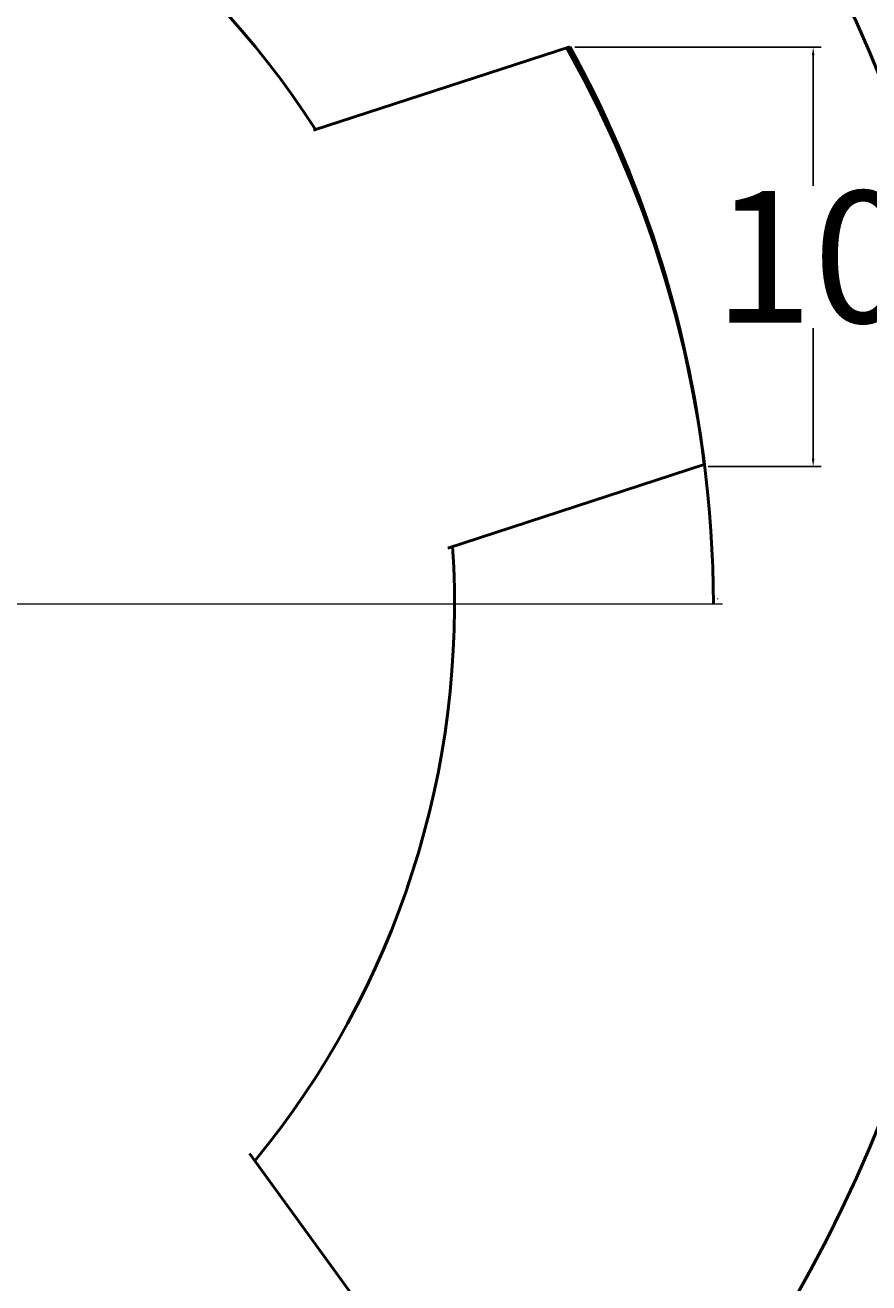
# Model space of a CAD drawing. Units: millimetres. Extents: x -50 to 109, y -46 to 152.
# Tile 6 of 18: x 9 to 29, y -22 to 6. Entities that reach past the tile are written whole.
import ezdxf

# ---------------------------------------------------------------- set-up
doc = ezdxf.new("R2010")
doc.units = ezdxf.units.MM
doc.header["$MEASUREMENT"] = 0
doc.linetypes.add('CENTER', pattern=[50.8, 31.75, -6.35, 6.35, -6.35])
for name, color, linetype, lineweight in [('M-CNTR', 1, 'CENTER', 18), ('M-DIMS', 2, 'Continuous', 25), ('M-OUTL', 7, 'Continuous', 50)]:
    doc.layers.add(name, color=color, linetype=linetype, lineweight=lineweight)
doc.styles.get("Standard").update_dxf_attribs({"font": 'arial.ttf'})
doc.dimstyles.get("Standard").update_dxf_attribs({"dimtxt": 0.18, "dimasz": 0.18, "dimexe": 0.18, "dimexo": 0.0625, "dimgap": 0.09, "dimtad": 0, "dimtih": 1, "dimtoh": 1, "dimdec": 4, "dimzin": 0, "dimdsep": 46, "dimtxsty": 'Standard', "dimcen": 0.09, "dimadec": 0, "dimazin": 0, "dimtfac": 1, "dimtdec": 4, "dimtofl": 0, "dimtmove": 0, "dimatfit": 3, "dimfxl": 1, "dimtolj": 1, "dimtzin": 0, "dimarcsym": 0})

# ---------------------------------------------------------------- blocks, each defined once
blk = doc.blocks.new('*U1')
for p, q in [((-5, 2.851), (-5, -3.294)), ((5, 2.824), (5, -3.323))]:
    blk.add_line(p, q)
blk.add_arc((-0.069, -22.677), 26, 78.7582, 100.9333)
blk = doc.blocks.new('*U2')
at = {"layer": 'M-OUTL', "color": 0, "linetype": 'ByBlock', "lineweight": -2, "transparency": 16777216}
for p, rotation in [((20.551, 0.185), 288), ((12.307, -25), 216)]:
    blk.add_blockref('*U1', p, dxfattribs=dict(at, rotation=rotation))
blk = doc.blocks.new('*U6')
at = {"layer": 'M-CNTR', "color": 0, "transparency": 16777216}
blk.add_line((5.2, 0), (26.12, 0), dxfattribs=at)
blk = doc.blocks.new('*D20')
at = {"layer": 'Defpoints', "color": 0, "transparency": 16777216}
for p in [(21.766, 5.813), (24.805, -3.739), (27.264, -3.739)]:
    blk.add_point(p, dxfattribs=at)
at = {"layer": 'M-DIMS', "color": 0, "lineweight": -2, "transparency": 16777216}
for p, q in [((21.828, 5.813), (27.444, 5.813)), ((27.264, 5.633), (27.264, 2.659)), ((27.264, -3.559), (27.264, -0.585)), ((24.868, -3.739), (27.444, -3.739))]:
    blk.add_line(p, q, dxfattribs=at)
at = {"layer": 'M-DIMS', "color": 0, "transparency": 16777216}
for points in [[(27.234, 5.633), (27.294, 5.633), (27.264, 5.813)], [(27.234, -3.559), (27.294, -3.559), (27.264, -3.739)]]:
    blk.add_solid(points, dxfattribs=at)
at = {"layer": 'M-DIMS', "color": 0, "transparency": 16777216, "insert": (27.264, 1.037), "char_height": 0.18, "attachment_point": 5}
blk.add_mtext('\\A1;{\\H16.66667x;10}', dxfattribs=at)
blk = doc.blocks.new('*D23')
at = {"layer": 'Defpoints', "color": 0, "transparency": 16777216}
for p in [(24.75, 12.317), (-26.598, -25.885)]:
    blk.add_point(p, dxfattribs=at)
at = {"layer": 'M-DIMS', "color": 0, "lineweight": -2, "transparency": 16777216}
for p, q in [((-1.014, -6.784), (-0.834, -6.784)), ((-0.924, -6.874), (-0.924, -6.694)), ((-30.604, -28.865), (-26.742, -25.992)), ((-30.784, -28.865), (-30.604, -28.865))]:
    blk.add_line(p, q, dxfattribs=at)
at = {"layer": 'M-DIMS', "color": 0, "transparency": 16777216}
blk.add_solid([(-26.76, -25.968), (-26.724, -26.016), (-26.598, -25.885)], dxfattribs=at)
at = {"layer": 'M-DIMS', "color": 0, "transparency": 16777216, "insert": (-34.648, -28.865), "char_height": 0.18, "attachment_point": 5}
blk.add_mtext('\\A1;{\\H16.66667x;%%C64}', dxfattribs=at)
blk = doc.blocks.new('*D29')
at = {"layer": 'Defpoints', "color": 0, "transparency": 16777216}
for p in [(21.684, 15.863), (-23.531, -29.431)]:
    blk.add_point(p, dxfattribs=at)
at = {"layer": 'M-DIMS', "color": 0, "lineweight": -2, "transparency": 16777216}
for p, q in [((-1.014, -6.784), (-0.834, -6.784)), ((-0.924, -6.874), (-0.924, -6.694)), ((-37.096, -43.02), (-23.658, -29.559)), ((-37.276, -43.02), (-37.096, -43.02))]:
    blk.add_line(p, q, dxfattribs=at)
at = {"layer": 'M-DIMS', "color": 0, "transparency": 16777216}
blk.add_solid([(-23.68, -29.537), (-23.637, -29.58), (-23.531, -29.431)], dxfattribs=at)
at = {"layer": 'M-DIMS', "color": 0, "transparency": 16777216, "insert": (-37.592, -43.02), "char_height": 0.18, "attachment_point": 5}
blk.add_mtext('\\A1;∅64', dxfattribs=at)

msp = doc.modelspace()

# ---------------------------------------------------------------- linework, layer by layer
at = {"layer": 'M-OUTL'}
msp.add_circle((-0.92366, -6.78396), 32, dxfattribs=at)
for centre, radius, start, end in [((-0.91099, -6.86447), 20, 32.692944, 75.356698), ((-1.00931, -6.9517), 26, 0.182484, 29.36911), ((-0.91099, -6.86447), 20, 320.576114, 3.737711), ((-0.92366, -6.86889), 26, 0.242431, 0.243801)]:
    msp.add_arc(centre, radius, start, end, dxfattribs=at)

# ---------------------------------------------------------------- block references
at = {"layer": 'M-CNTR'}
msp.add_blockref('*U6', (-0.92366, -6.86889), dxfattribs=at)
at = {"layer": 'M-OUTL'}
msp.add_blockref('*U2', (0, 0), dxfattribs=at)

# ---------------------------------------------------------------- dimensions: what is measured, and where the dimension line sits
at = {"layer": 'M-DIMS'}
dim = msp.add_diameter_dim_2p(p1=(21.68387, 15.86332), p2=(-23.53119, -29.43125), dimstyle='Standard', override={"dimdec": 0, "dimlfac": 1, "dimrnd": 0, "dimzin": 0, "dimdsep": 46, "dimlunit": 2}, dxfattribs=at)
dim.commit()
dim.dimension.update_dxf_attribs({"geometry": '*D29', "text_midpoint": (-37.59218, -43.01962), "dimtype": 163})
dim = msp.add_diameter_dim_2p(p1=(24.75033, 12.31698), p2=(-26.59765, -25.88491), text='{\\H16.66667x;%%C64}', dimstyle='Standard', override={"dimclrd": 0, "dimclre": 0, "dimclrt": 0}, dxfattribs=at)
dim.commit()
dim.dimension.update_dxf_attribs({"geometry": '*D23', "text_midpoint": (-34.64806, -28.86518), "dimtype": 163})
dim = msp.add_linear_dim(base=(27.26425, -3.73924), p1=(21.76599, 5.81281), p2=(24.80523, -3.73924), angle=90, text='{\\H16.66667x;10}', dimstyle='Standard', override={"dimclrd": 0, "dimclre": 0, "dimclrt": 0}, dxfattribs=at)
dim.commit()
dim.dimension.update_dxf_attribs({"geometry": '*D20', "text_midpoint": (27.26425, 1.03679)})

doc.saveas('drawing.dxf')
